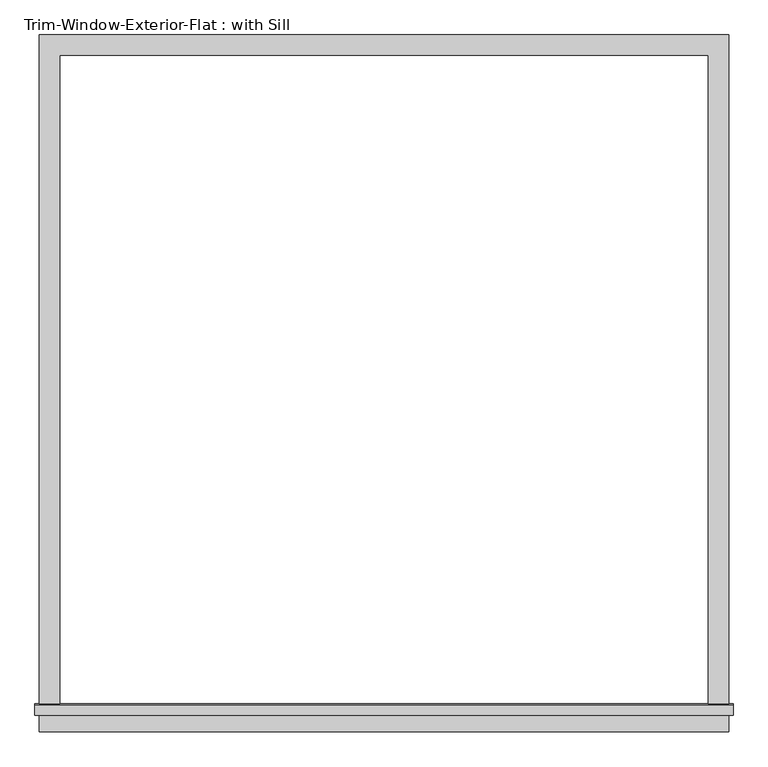
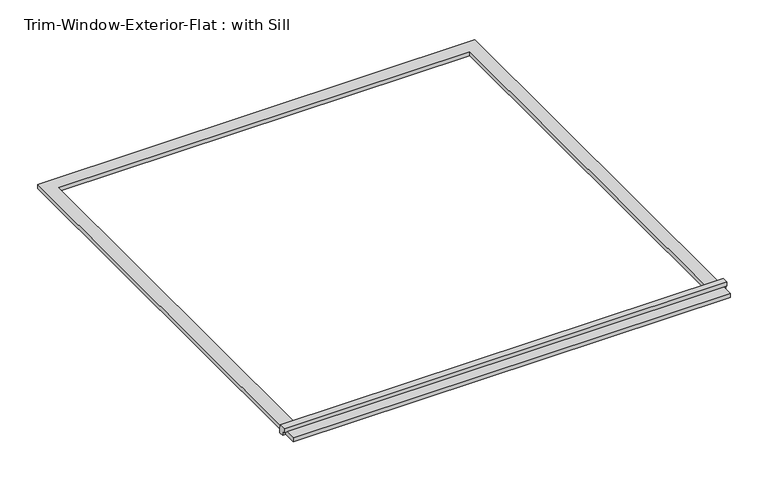
"""IFC4 building model written with IfcOpenShell, lengths in millimetres: proxy geometry, Trim-Window-Exterior-Flat : with Sill."""

from ifc_helpers import new_model, si_unit, frame, origin, origin_with_axes, place, context, project, spatial, polyline, outline, extrude, source, transform, mapped, element, save


def trim_window_exterior_flat_with_sill_b601e94a(model_context):
    return source(origin(), model_context, "Body", "SweptSolid", [
        extrude(outline(polyline([(971.55, -1850.9823709), (971.55, -1908.1323709), (-971.55, -1908.1323709), (-971.55, -1850.9823709), (971.55, -1850.9823709)])), origin_with_axes(), (0.0, 0.0, 1.0), 19.05),
        extrude(outline(polyline([(-1860.55, 38.1), (-1831.2580645, 38.1), (-1828.8, 19.05), (-1828.8, 0.0), (-1850.9823709, 0.0), (-1850.9823709, 19.05), (-1860.55, 19.05), (-1860.55, 38.1)])), frame((-984.25, 0.0, 0.0), z_axis=(1.0, 0.0, 0.0), x_axis=(0.0, 1.0, 0.0)), (0.0, 0.0, 1.0), 1968.5),
        extrude(outline(polyline([(-971.55, 57.15), (971.55, 57.15), (971.55, -1828.8), (914.4, -1828.8), (914.4, 0.0), (-914.4, 0.0), (-914.4, -1828.8), (-971.55, -1828.8), (-971.55, 57.15)])), origin_with_axes(), (0.0, 0.0, 1.0), 19.05),
    ])


if __name__ == "__main__":
    model = new_model("IFC4")
    model_context = context("Model", 3, world=origin())
    ifc_project = project(units=[si_unit("LENGTHUNIT", "METRE", prefix="MILLI")], contexts=[model_context])
    site = spatial("IfcSite", under=ifc_project)
    building = spatial("IfcBuilding", under=site)
    placement = place(None, origin())
    trim_window_exterior_flat_with_sill_shape = trim_window_exterior_flat_with_sill_b601e94a(model_context)
    element("IfcBuildingElementProxy", 1, Name="Trim-Window-Exterior-Flat : with Sill", ObjectType="Trim-Window-Exterior-Flat : with Sill", at=placement, inside=building, context=model_context, shape_type="MappedRepresentation", body=[
        mapped(trim_window_exterior_flat_with_sill_shape, transform((0.0, 0.0, 0.0), x_axis=(1.0, 0.0, 0.0), y_axis=(0.0, 1.0, 0.0), z_axis=(0.0, 0.0, 1.0))),
    ])
    save(model, "model.ifc")

# Revit data of these elements
# Type "Trim-Window-Exterior-Flat : with Sill"
#   Trim Width = 0' - 2 1/4"
#   Trim Thickness_Picture Frame = 0' - 1 1/4"
#   Trim Thickness_with Sill = 0' - 0 3/4"
#   Sill Thickness = 0' - 1 1/4"
#   Opening Width [instance default] = 2' - 0"
#   Opening Height [instance default] = 3' - 0"
#   Default Elevation = 4' - 0"
#   Sill = yes
#   Picture Frame = no
#   Trim Material [instance default] = none
# Element 1 (IfcBuildingElementProxy, "Trim-Window-Exterior-Flat : with Sill")
#   Opening Width = 6' - 0"
#   Opening Height = 6' - 0"
#   Trim Material = Clad - White
#   Materials on its faces: "Clad - White"
# Materials
#   "Clad - White": class "Wood", colour RGB 242 242 238, transparency 0, Cost = 0
